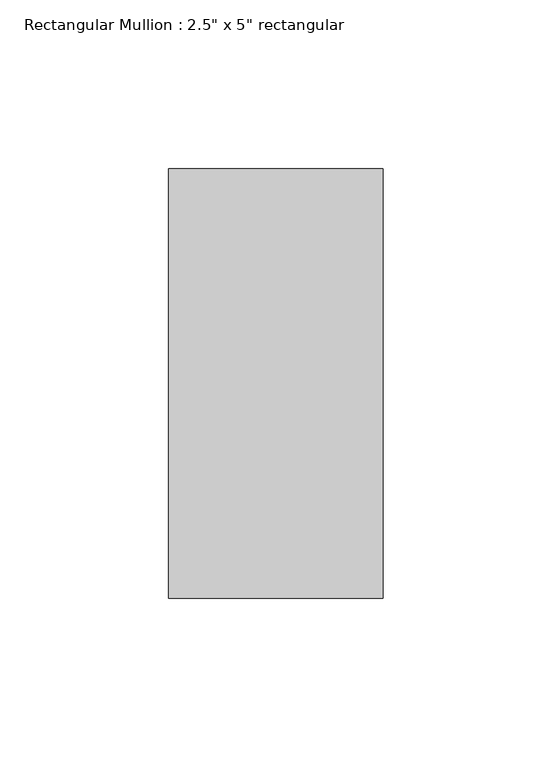
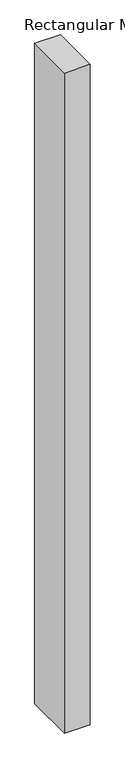
"""IFC4 building model written with IfcOpenShell, lengths in millimetres: member geometry."""

from ifc_helpers import new_model, si_unit, frame, origin, place, context, project, spatial, polyline, outline, extrude, source, transform, mapped, element, save


def member_6515f0de(model_context):
    return source(origin(), model_context, "Body", "SweptSolid", [
        extrude(outline(polyline([(31.75, 63.5), (31.75, -63.5), (-31.75, -63.5), (-31.75, 63.5), (31.75, 63.5)])), frame((0.0, 0.0, -1718.7125392), z_axis=(0.0, 0.0, 1.0), x_axis=(1.0, 0.0, 0.0)), (0.0, 0.0, 1.0), 1718.7125392),
    ])


if __name__ == "__main__":
    model = new_model("IFC4")
    model_context = context("Model", 3, world=origin())
    ifc_project = project(units=[si_unit("LENGTHUNIT", "METRE", prefix="MILLI")], contexts=[model_context])
    site = spatial("IfcSite", under=ifc_project)
    building = spatial("IfcBuilding", under=site)
    placement = place(None, origin())
    member_shape = member_6515f0de(model_context)
    element("IfcMember", 1, ObjectType="Rectangular Mullion : 2.5\" x 5\" rectangular", at=placement, inside=building, context=model_context, shape_type="MappedRepresentation", body=[
        mapped(member_shape, transform((0.0, 0.0, 0.0), x_axis=(1.0, 0.0, 0.0), y_axis=(0.0, 1.0, 0.0), z_axis=(0.0, 0.0, 1.0))),
    ])
    save(model, "model.ifc")

# Revit data of these elements
# Type "Rectangular Mullion : 2.5\" x 5\" rectangular"
#   built-in parameter 1007304 = 0.416667 (stored number, unit not read)
#   built-in parameter 1007301 = 0.104167 (stored number, unit not read)
#   built-in parameter 1007300 = 0.104167 (stored number, unit not read)
# Element 1 (IfcMember, "Rectangular Mullion : 2.5\" x 5\" rectangular")
#   Materials on its faces: "Aluminum"
# Materials
#   "Aluminum": class "Metal", colour RGB 247 247 247, transparency 0, Description = "Aluminum 6061", Cost = 0
